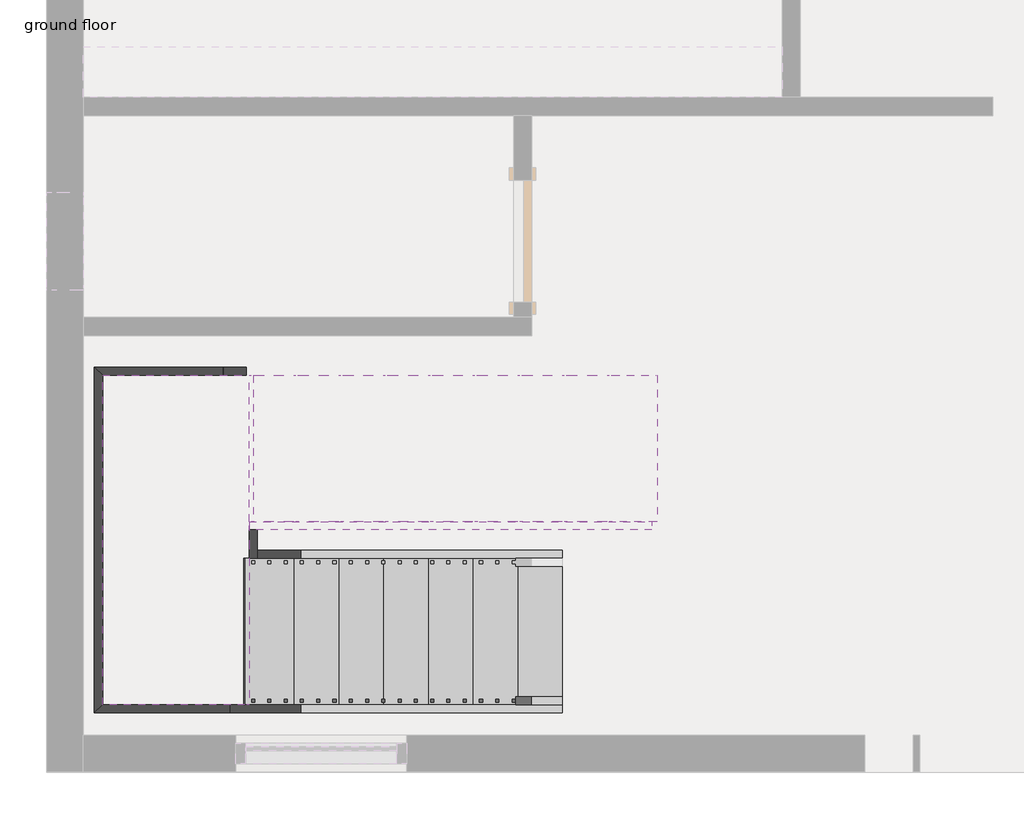
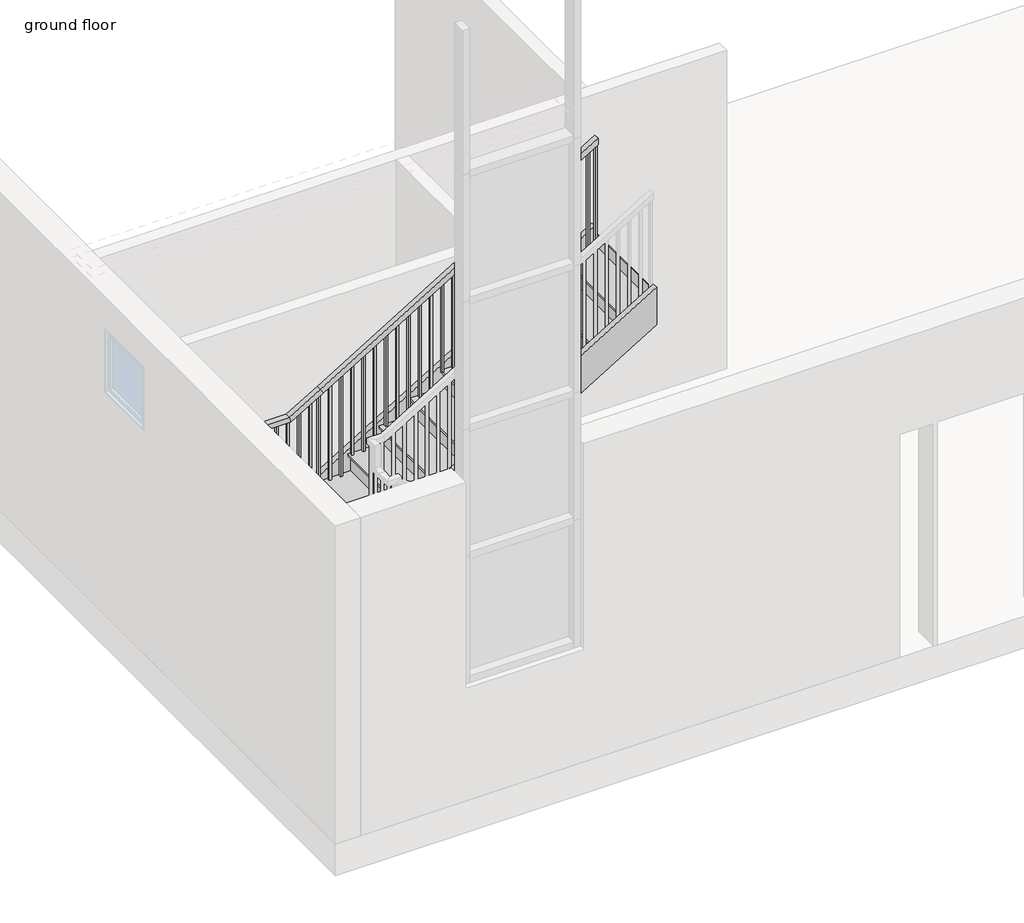
# One storey, part 3 of 3: 8 members, 2 stair flights, 1 railing, 1 slab.
"""IFC4 building model written with IfcOpenShell, lengths in millimetres."""

from ifc_helpers import new_model, si_unit, frame, origin, place, context, project, spatial, polyline, outline, extrude, faceted_brep, transform, mapped, element, save
from components import non_monolithic_landing_1e1f2eae, stair_flight_155d8820, stair_flight_d3a95e7b

model = new_model("IFC4")

# Units and contexts
model_context = context("Model", 3, world=origin())
ifc_project = project(units=[si_unit("LENGTHUNIT", "METRE", prefix="MILLI")], contexts=[model_context])

# Site, building, storey
site = spatial("IfcSite", under=ifc_project)
building = spatial("IfcBuilding", under=site)
storey = spatial("IfcBuildingStorey", under=building, Name="ground floor", Elevation=304.8)

# Members
placement = place(None, origin())
element("IfcMember", 1, ObjectType="Stringer - 2\" Width", at=placement, inside=storey, context=model_context, shape_type="SweptSolid", body=[
    extrude(outline(polyline([(304.8, -12620.1777023), (516.914512, -12620.1777023), (1735.6666667, -14631.1187576), (1430.8666667, -14716.2732141), (304.8, -12858.2632141), (304.8, -12620.1777023)])), frame((0.0, -405.7320925, 0.0), z_axis=(0.0, 1.0, 0.0), x_axis=(0.0, 0.0, 1.0)), (0.0, 0.0, 1.0), 50.8),
])
element("IfcMember", 2, ObjectType="Stringer - 2\" Width", at=placement, inside=storey, context=model_context, shape_type="SweptSolid", body=[
    extrude(outline(polyline([(304.8, -12620.1777023), (516.914512, -12620.1777023), (1671.4599665, -14525.1777023), (1315.051205, -14525.1777023), (304.8, -12858.2632141), (304.8, -12620.1777023)])), frame((0.0, 559.4679075, 0.0), z_axis=(0.0, 1.0, 0.0), x_axis=(0.0, 0.0, 1.0)), (0.0, 0.0, 1.0), 50.8),
])
element("IfcMember", 3, ObjectType="Stringer - 2\" Width", at=placement, inside=storey, context=model_context, shape_type="SweptSolid", body=[
    extrude(outline(polyline([(1735.6666667, -14800.2366471), (1430.8666667, -14715.0821905), (3039.1724171, -12061.3777023), (3395.5811786, -12061.3777023), (1735.6666667, -14800.2366471)])), frame((0.0, 1702.4679075, 0.0), z_axis=(0.0, 1.0, 0.0), x_axis=(0.0, 0.0, 1.0)), (0.0, 0.0, 1.0), 50.8),
])
element("IfcMember", 4, ObjectType="Stringer - 2\" Width", at=placement, inside=storey, context=model_context, shape_type="SweptSolid", body=[
    extrude(outline(polyline([(1871.5811786, -14575.9777023), (1515.1724171, -14575.9777023), (3039.1724171, -12061.3777023), (3395.5811786, -12061.3777023), (1871.5811786, -14575.9777023)])), frame((0.0, 737.2679075, 0.0), z_axis=(0.0, 1.0, 0.0), x_axis=(0.0, 0.0, 1.0)), (0.0, 0.0, 1.0), 50.8),
])
element("IfcMember", 5, ObjectType="Stringer - 2\" Width", at=placement, inside=storey, context=model_context, shape_type="Brep", body=[
    faceted_brep([(-14800.2366471, 1702.4679075, 1735.6666667), (-14800.2366471, 1753.2679075, 1735.6666667), (-15541.1777023, 1753.2679075, 1735.6666667), (-15490.3777023, 1702.4679075, 1735.6666667), (-14715.0821905, 1702.4679075, 1430.8666667), (-15490.3777023, 1702.4679075, 1430.8666667), (-14715.0821905, 1753.2679075, 1430.8666667), (-15541.1777023, 1753.2679075, 1430.8666667)], [[[0, 1, 2, 3]], [[4, 0, 3, 5]], [[6, 4, 5, 7]], [[1, 6, 7, 2]], [[1, 0, 4, 6]], [[2, 7, 5, 3]]]),
])
element("IfcMember", 6, ObjectType="Stringer - 2\" Width", at=placement, inside=storey, context=model_context, shape_type="SweptSolid", body=[
    extrude(outline(polyline([(-15541.1777023, 1753.2679075), (-15490.3777023, 1702.4679075), (-15490.3777023, -354.9320925), (-15541.1777023, -405.7320925), (-15541.1777023, 1753.2679075)])), frame((0.0, 0.0, 1430.8666667), z_axis=(0.0, 0.0, 1.0), x_axis=(1.0, 0.0, 0.0)), (0.0, 0.0, 1.0), 304.8),
])
element("IfcMember", 7, ObjectType="Stringer - 2\" Width", at=placement, inside=storey, context=model_context, shape_type="Brep", body=[
    faceted_brep([(-15490.3777023, -354.9320925, 1735.6666667), (-15541.1777023, -405.7320925, 1735.6666667), (-14631.1187576, -405.7320925, 1735.6666667), (-14631.1187576, -354.9320925, 1735.6666667), (-15490.3777023, -354.9320925, 1430.8666667), (-14716.2732141, -354.9320925, 1430.8666667), (-15541.1777023, -405.7320925, 1430.8666667), (-14716.2732141, -405.7320925, 1430.8666667)], [[[0, 1, 2, 3]], [[4, 0, 3, 5]], [[6, 4, 5, 7]], [[1, 6, 7, 2]], [[1, 0, 4, 6]], [[2, 7, 5, 3]]]),
])
element("IfcMember", 8, ObjectType="Stringer - 2\" Width", at=placement, inside=storey, context=model_context, shape_type="SweptSolid", body=[
    extrude(outline(polyline([(-14525.1777023, 559.4679075), (-14575.9777023, 559.4679075), (-14575.9777023, 737.2679075), (-14525.1777023, 737.2679075), (-14525.1777023, 559.4679075)])), frame((0.0, 0.0, 1430.8666667), z_axis=(0.0, 0.0, 1.0), x_axis=(1.0, 0.0, 0.0)), (0.0, 0.0, 1.0), 304.8),
])

# Railing
element("IfcRailing", 9, ObjectType="Handrail - Rectangular", at=placement, inside=storey, context=model_context, shape_type="SolidModel", body=[
    faceted_brep([(-12620.1777023, -354.9320925, 1388.5333333), (-12620.1777023, -354.9320925, 1329.1318731), (-12620.1777023, -304.1320925, 1329.1318731), (-12620.1777023, -304.1320925, 1388.5333333), (-14575.9777023, -354.9320925, 2573.8666667), (-14590.1701117, -354.9320925, 2523.0666667), (-14590.1701117, -304.1320925, 2523.0666667), (-14575.9777023, -304.1320925, 2573.8666667), (-15490.3777023, -354.9320925, 2573.8666667), (-15490.3777023, -354.9320925, 2523.0666667), (-15439.5777023, -304.1320925, 2523.0666667), (-15439.5777023, -304.1320925, 2573.8666667), (-15490.3777023, 1702.4679075, 2573.8666667), (-15490.3777023, 1702.4679075, 2523.0666667), (-15439.5777023, 1651.6679075, 2523.0666667), (-15439.5777023, 1651.6679075, 2573.8666667), (-14855.3777023, 1702.4679075, 2573.8666667), (-14841.1852929, 1702.4679075, 2523.0666667), (-14841.1852929, 1651.6679075, 2523.0666667), (-14855.3777023, 1651.6679075, 2573.8666667), (-14575.9777023, 1702.4679075, 2743.2), (-14549.6479751, 1702.4679075, 2699.7559502), (-14549.6479751, 1651.6679075, 2699.7559502), (-14575.9777023, 1651.6679075, 2743.2), (-12061.3777023, 1702.4679075, 4267.2), (-12061.3777023, 1651.6679075, 4267.2), (-12061.3777023, 1651.6679075, 4207.7985397), (-12061.3777023, 1702.4679075, 4207.7985397)], [[[0, 1, 2, 3]], [[1, 0, 4, 5]], [[2, 1, 5, 6]], [[3, 2, 6, 7]], [[0, 3, 7, 4]], [[5, 4, 8, 9]], [[6, 5, 9, 10]], [[7, 6, 10, 11]], [[4, 7, 11, 8]], [[9, 8, 12, 13]], [[10, 9, 13, 14]], [[11, 10, 14, 15]], [[8, 11, 15, 12]], [[13, 12, 16, 17]], [[14, 13, 17, 18]], [[15, 14, 18, 19]], [[12, 15, 19, 16]], [[17, 16, 20, 21]], [[18, 17, 21, 22]], [[19, 18, 22, 23]], [[16, 19, 23, 20]], [[24, 25, 26, 27]], [[21, 20, 24, 27]], [[22, 21, 27, 26]], [[23, 22, 26, 25]], [[20, 23, 25, 24]]]),
    extrude(outline(polyline([(4155.8439943, -12147.1027023), (3183.4666667, -12147.1027023), (3183.4666667, -12128.0527023), (4167.3894488, -12128.0527023), (4155.8439943, -12147.1027023)])), frame((0.0, 1667.5429075, 0.0), z_axis=(0.0, 1.0, 0.0), x_axis=(0.0, 0.0, 1.0)), (0.0, 0.0, 1.0), 19.05),
    extrude(outline(polyline([(4094.2682367, -12248.7027023), (3183.4666667, -12248.7027023), (3183.4666667, -12229.6527023), (4105.8136913, -12229.6527023), (4094.2682367, -12248.7027023)])), frame((0.0, 1667.5429075, 0.0), z_axis=(0.0, 1.0, 0.0), x_axis=(0.0, 0.0, 1.0)), (0.0, 0.0, 1.0), 19.05),
    extrude(outline(polyline([(4032.6924791, -12350.3027023), (3183.4666667, -12350.3027023), (3183.4666667, -12331.2527023), (4044.2379337, -12331.2527023), (4032.6924791, -12350.3027023)])), frame((0.0, 1667.5429075, 0.0), z_axis=(0.0, 1.0, 0.0), x_axis=(0.0, 0.0, 1.0)), (0.0, 0.0, 1.0), 19.05),
    extrude(outline(polyline([(3971.1167216, -12451.9027023), (3014.1333333, -12451.9027023), (3014.1333333, -12432.8527023), (3982.6621761, -12432.8527023), (3971.1167216, -12451.9027023)])), frame((0.0, 1667.5429075, 0.0), z_axis=(0.0, 1.0, 0.0), x_axis=(0.0, 0.0, 1.0)), (0.0, 0.0, 1.0), 19.05),
    extrude(outline(polyline([(3909.540964, -12553.5027023), (3014.1333333, -12553.5027023), (3014.1333333, -12534.4527023), (3921.0864185, -12534.4527023), (3909.540964, -12553.5027023)])), frame((0.0, 1667.5429075, 0.0), z_axis=(0.0, 1.0, 0.0), x_axis=(0.0, 0.0, 1.0)), (0.0, 0.0, 1.0), 19.05),
    extrude(outline(polyline([(3847.9652064, -12655.1027023), (2844.8, -12655.1027023), (2844.8, -12636.0527023), (3859.510661, -12636.0527023), (3847.9652064, -12655.1027023)])), frame((0.0, 1667.5429075, 0.0), z_axis=(0.0, 1.0, 0.0), x_axis=(0.0, 0.0, 1.0)), (0.0, 0.0, 1.0), 19.05),
    extrude(outline(polyline([(3786.3894488, -12756.7027023), (2844.8, -12756.7027023), (2844.8, -12737.6527023), (3797.9349034, -12737.6527023), (3786.3894488, -12756.7027023)])), frame((0.0, 1667.5429075, 0.0), z_axis=(0.0, 1.0, 0.0), x_axis=(0.0, 0.0, 1.0)), (0.0, 0.0, 1.0), 19.05),
    extrude(outline(polyline([(3724.8136913, -12858.3027023), (2844.8, -12858.3027023), (2844.8, -12839.2527023), (3736.3591458, -12839.2527023), (3724.8136913, -12858.3027023)])), frame((0.0, 1667.5429075, 0.0), z_axis=(0.0, 1.0, 0.0), x_axis=(0.0, 0.0, 1.0)), (0.0, 0.0, 1.0), 19.05),
    extrude(outline(polyline([(3663.2379337, -12959.9027023), (2675.4666667, -12959.9027023), (2675.4666667, -12940.8527023), (3674.7833882, -12940.8527023), (3663.2379337, -12959.9027023)])), frame((0.0, 1667.5429075, 0.0), z_axis=(0.0, 1.0, 0.0), x_axis=(0.0, 0.0, 1.0)), (0.0, 0.0, 1.0), 19.05),
    extrude(outline(polyline([(3601.6621761, -13061.5027023), (2675.4666667, -13061.5027023), (2675.4666667, -13042.4527023), (3613.2076307, -13042.4527023), (3601.6621761, -13061.5027023)])), frame((0.0, 1667.5429075, 0.0), z_axis=(0.0, 1.0, 0.0), x_axis=(0.0, 0.0, 1.0)), (0.0, 0.0, 1.0), 19.05),
    extrude(outline(polyline([(3540.0864185, -13163.1027023), (2675.4666667, -13163.1027023), (2675.4666667, -13144.0527023), (3551.6318731, -13144.0527023), (3540.0864185, -13163.1027023)])), frame((0.0, 1667.5429075, 0.0), z_axis=(0.0, 1.0, 0.0), x_axis=(0.0, 0.0, 1.0)), (0.0, 0.0, 1.0), 19.05),
    extrude(outline(polyline([(3478.510661, -13264.7027023), (2506.1333333, -13264.7027023), (2506.1333333, -13245.6527023), (3490.0561155, -13245.6527023), (3478.510661, -13264.7027023)])), frame((0.0, 1667.5429075, 0.0), z_axis=(0.0, 1.0, 0.0), x_axis=(0.0, 0.0, 1.0)), (0.0, 0.0, 1.0), 19.05),
    extrude(outline(polyline([(3416.9349034, -13366.3027023), (2506.1333333, -13366.3027023), (2506.1333333, -13347.2527023), (3428.4803579, -13347.2527023), (3416.9349034, -13366.3027023)])), frame((0.0, 1667.5429075, 0.0), z_axis=(0.0, 1.0, 0.0), x_axis=(0.0, 0.0, 1.0)), (0.0, 0.0, 1.0), 19.05),
    extrude(outline(polyline([(3355.3591458, -13467.9027023), (2506.1333333, -13467.9027023), (2506.1333333, -13448.8527023), (3366.9046004, -13448.8527023), (3355.3591458, -13467.9027023)])), frame((0.0, 1667.5429075, 0.0), z_axis=(0.0, 1.0, 0.0), x_axis=(0.0, 0.0, 1.0)), (0.0, 0.0, 1.0), 19.05),
    extrude(outline(polyline([(3293.7833882, -13569.5027023), (2336.8, -13569.5027023), (2336.8, -13550.4527023), (3305.3288428, -13550.4527023), (3293.7833882, -13569.5027023)])), frame((0.0, 1667.5429075, 0.0), z_axis=(0.0, 1.0, 0.0), x_axis=(0.0, 0.0, 1.0)), (0.0, 0.0, 1.0), 19.05),
    extrude(outline(polyline([(3232.2076307, -13671.1027023), (2336.8, -13671.1027023), (2336.8, -13652.0527023), (3243.7530852, -13652.0527023), (3232.2076307, -13671.1027023)])), frame((0.0, 1667.5429075, 0.0), z_axis=(0.0, 1.0, 0.0), x_axis=(0.0, 0.0, 1.0)), (0.0, 0.0, 1.0), 19.05),
    extrude(outline(polyline([(3170.6318731, -13772.7027023), (2167.4666667, -13772.7027023), (2167.4666667, -13753.6527023), (3182.1773276, -13753.6527023), (3170.6318731, -13772.7027023)])), frame((0.0, 1667.5429075, 0.0), z_axis=(0.0, 1.0, 0.0), x_axis=(0.0, 0.0, 1.0)), (0.0, 0.0, 1.0), 19.05),
    extrude(outline(polyline([(3109.0561155, -13874.3027023), (2167.4666667, -13874.3027023), (2167.4666667, -13855.2527023), (3120.60157, -13855.2527023), (3109.0561155, -13874.3027023)])), frame((0.0, 1667.5429075, 0.0), z_axis=(0.0, 1.0, 0.0), x_axis=(0.0, 0.0, 1.0)), (0.0, 0.0, 1.0), 19.05),
    extrude(outline(polyline([(3047.4803579, -13975.9027023), (2167.4666667, -13975.9027023), (2167.4666667, -13956.8527023), (3059.0258125, -13956.8527023), (3047.4803579, -13975.9027023)])), frame((0.0, 1667.5429075, 0.0), z_axis=(0.0, 1.0, 0.0), x_axis=(0.0, 0.0, 1.0)), (0.0, 0.0, 1.0), 19.05),
    extrude(outline(polyline([(2985.9046004, -14077.5027023), (1998.1333333, -14077.5027023), (1998.1333333, -14058.4527023), (2997.4500549, -14058.4527023), (2985.9046004, -14077.5027023)])), frame((0.0, 1667.5429075, 0.0), z_axis=(0.0, 1.0, 0.0), x_axis=(0.0, 0.0, 1.0)), (0.0, 0.0, 1.0), 19.05),
    extrude(outline(polyline([(2924.3288428, -14179.1027023), (1998.1333333, -14179.1027023), (1998.1333333, -14160.0527023), (2935.8742973, -14160.0527023), (2924.3288428, -14179.1027023)])), frame((0.0, 1667.5429075, 0.0), z_axis=(0.0, 1.0, 0.0), x_axis=(0.0, 0.0, 1.0)), (0.0, 0.0, 1.0), 19.05),
    extrude(outline(polyline([(2862.7530852, -14280.7027023), (1998.1333333, -14280.7027023), (1998.1333333, -14261.6527023), (2874.2985397, -14261.6527023), (2862.7530852, -14280.7027023)])), frame((0.0, 1667.5429075, 0.0), z_axis=(0.0, 1.0, 0.0), x_axis=(0.0, 0.0, 1.0)), (0.0, 0.0, 1.0), 19.05),
    extrude(outline(polyline([(2801.1773276, -14382.3027023), (1828.8, -14382.3027023), (1828.8, -14363.2527023), (2812.7227822, -14363.2527023), (2801.1773276, -14382.3027023)])), frame((0.0, 1667.5429075, 0.0), z_axis=(0.0, 1.0, 0.0), x_axis=(0.0, 0.0, 1.0)), (0.0, 0.0, 1.0), 19.05),
    extrude(outline(polyline([(2739.60157, -14483.9027023), (1828.8, -14483.9027023), (1828.8, -14464.8527023), (2751.1470246, -14464.8527023), (2739.60157, -14483.9027023)])), frame((0.0, 1667.5429075, 0.0), z_axis=(0.0, 1.0, 0.0), x_axis=(0.0, 0.0, 1.0)), (0.0, 0.0, 1.0), 19.05),
    extrude(outline(polyline([(2631.8439943, -14661.7027023), (1659.4666667, -14661.7027023), (1659.4666667, -14642.6527023), (2643.3894488, -14642.6527023), (2631.8439943, -14661.7027023)])), frame((0.0, 1667.5429075, 0.0), z_axis=(0.0, 1.0, 0.0), x_axis=(0.0, 0.0, 1.0)), (0.0, 0.0, 1.0), 19.05),
    extrude(outline(polyline([(2570.2682367, -14763.3027023), (1659.4666667, -14763.3027023), (1659.4666667, -14744.2527023), (2581.8136913, -14744.2527023), (2570.2682367, -14763.3027023)])), frame((0.0, 1667.5429075, 0.0), z_axis=(0.0, 1.0, 0.0), x_axis=(0.0, 0.0, 1.0)), (0.0, 0.0, 1.0), 19.05),
    extrude(outline(polyline([(-14864.9027023, 1686.5929075), (-14845.8527023, 1686.5929075), (-14845.8527023, 1667.5429075), (-14864.9027023, 1667.5429075), (-14864.9027023, 1686.5929075)])), frame((0.0, 0.0, 1659.4666667), z_axis=(0.0, 0.0, 1.0), x_axis=(1.0, 0.0, 0.0)), (0.0, 0.0, 1.0), 863.6),
    extrude(outline(polyline([(-14966.5027023, 1686.5929075), (-14947.4527023, 1686.5929075), (-14947.4527023, 1667.5429075), (-14966.5027023, 1667.5429075), (-14966.5027023, 1686.5929075)])), frame((0.0, 0.0, 1659.4666667), z_axis=(0.0, 0.0, 1.0), x_axis=(1.0, 0.0, 0.0)), (0.0, 0.0, 1.0), 863.6),
    extrude(outline(polyline([(-15068.1027023, 1686.5929075), (-15049.0527023, 1686.5929075), (-15049.0527023, 1667.5429075), (-15068.1027023, 1667.5429075), (-15068.1027023, 1686.5929075)])), frame((0.0, 0.0, 1659.4666667), z_axis=(0.0, 0.0, 1.0), x_axis=(1.0, 0.0, 0.0)), (0.0, 0.0, 1.0), 863.6),
    extrude(outline(polyline([(-15169.7027023, 1686.5929075), (-15150.6527023, 1686.5929075), (-15150.6527023, 1667.5429075), (-15169.7027023, 1667.5429075), (-15169.7027023, 1686.5929075)])), frame((0.0, 0.0, 1659.4666667), z_axis=(0.0, 0.0, 1.0), x_axis=(1.0, 0.0, 0.0)), (0.0, 0.0, 1.0), 863.6),
    extrude(outline(polyline([(-15271.3027023, 1686.5929075), (-15252.2527023, 1686.5929075), (-15252.2527023, 1667.5429075), (-15271.3027023, 1667.5429075), (-15271.3027023, 1686.5929075)])), frame((0.0, 0.0, 1659.4666667), z_axis=(0.0, 0.0, 1.0), x_axis=(1.0, 0.0, 0.0)), (0.0, 0.0, 1.0), 863.6),
    extrude(outline(polyline([(-15372.9027023, 1686.5929075), (-15353.8527023, 1686.5929075), (-15353.8527023, 1667.5429075), (-15372.9027023, 1667.5429075), (-15372.9027023, 1686.5929075)])), frame((0.0, 0.0, 1659.4666667), z_axis=(0.0, 0.0, 1.0), x_axis=(1.0, 0.0, 0.0)), (0.0, 0.0, 1.0), 863.6),
    extrude(outline(polyline([(-15474.5027023, 1591.3429075), (-15474.5027023, 1610.3929075), (-15455.4527023, 1610.3929075), (-15455.4527023, 1591.3429075), (-15474.5027023, 1591.3429075)])), frame((0.0, 0.0, 1659.4666667), z_axis=(0.0, 0.0, 1.0), x_axis=(1.0, 0.0, 0.0)), (0.0, 0.0, 1.0), 863.6),
    extrude(outline(polyline([(-15474.5027023, 1489.7429075), (-15474.5027023, 1508.7929075), (-15455.4527023, 1508.7929075), (-15455.4527023, 1489.7429075), (-15474.5027023, 1489.7429075)])), frame((0.0, 0.0, 1659.4666667), z_axis=(0.0, 0.0, 1.0), x_axis=(1.0, 0.0, 0.0)), (0.0, 0.0, 1.0), 863.6),
    extrude(outline(polyline([(-15474.5027023, 1388.1429075), (-15474.5027023, 1407.1929075), (-15455.4527023, 1407.1929075), (-15455.4527023, 1388.1429075), (-15474.5027023, 1388.1429075)])), frame((0.0, 0.0, 1659.4666667), z_axis=(0.0, 0.0, 1.0), x_axis=(1.0, 0.0, 0.0)), (0.0, 0.0, 1.0), 863.6),
    extrude(outline(polyline([(-15474.5027023, 1286.5429075), (-15474.5027023, 1305.5929075), (-15455.4527023, 1305.5929075), (-15455.4527023, 1286.5429075), (-15474.5027023, 1286.5429075)])), frame((0.0, 0.0, 1659.4666667), z_axis=(0.0, 0.0, 1.0), x_axis=(1.0, 0.0, 0.0)), (0.0, 0.0, 1.0), 863.6),
    extrude(outline(polyline([(-15474.5027023, 1184.9429075), (-15474.5027023, 1203.9929075), (-15455.4527023, 1203.9929075), (-15455.4527023, 1184.9429075), (-15474.5027023, 1184.9429075)])), frame((0.0, 0.0, 1659.4666667), z_axis=(0.0, 0.0, 1.0), x_axis=(1.0, 0.0, 0.0)), (0.0, 0.0, 1.0), 863.6),
    extrude(outline(polyline([(-15474.5027023, 1083.3429075), (-15474.5027023, 1102.3929075), (-15455.4527023, 1102.3929075), (-15455.4527023, 1083.3429075), (-15474.5027023, 1083.3429075)])), frame((0.0, 0.0, 1659.4666667), z_axis=(0.0, 0.0, 1.0), x_axis=(1.0, 0.0, 0.0)), (0.0, 0.0, 1.0), 863.6),
    extrude(outline(polyline([(-15474.5027023, 981.7429075), (-15474.5027023, 1000.7929075), (-15455.4527023, 1000.7929075), (-15455.4527023, 981.7429075), (-15474.5027023, 981.7429075)])), frame((0.0, 0.0, 1659.4666667), z_axis=(0.0, 0.0, 1.0), x_axis=(1.0, 0.0, 0.0)), (0.0, 0.0, 1.0), 863.6),
    extrude(outline(polyline([(-15474.5027023, 880.1429075), (-15474.5027023, 899.1929075), (-15455.4527023, 899.1929075), (-15455.4527023, 880.1429075), (-15474.5027023, 880.1429075)])), frame((0.0, 0.0, 1659.4666667), z_axis=(0.0, 0.0, 1.0), x_axis=(1.0, 0.0, 0.0)), (0.0, 0.0, 1.0), 863.6),
    extrude(outline(polyline([(-15474.5027023, 778.5429075), (-15474.5027023, 797.5929075), (-15455.4527023, 797.5929075), (-15455.4527023, 778.5429075), (-15474.5027023, 778.5429075)])), frame((0.0, 0.0, 1659.4666667), z_axis=(0.0, 0.0, 1.0), x_axis=(1.0, 0.0, 0.0)), (0.0, 0.0, 1.0), 863.6),
    extrude(outline(polyline([(-15474.5027023, 676.9429075), (-15474.5027023, 695.9929075), (-15455.4527023, 695.9929075), (-15455.4527023, 676.9429075), (-15474.5027023, 676.9429075)])), frame((0.0, 0.0, 1659.4666667), z_axis=(0.0, 0.0, 1.0), x_axis=(1.0, 0.0, 0.0)), (0.0, 0.0, 1.0), 863.6),
    extrude(outline(polyline([(-15474.5027023, 575.3429075), (-15474.5027023, 594.3929075), (-15455.4527023, 594.3929075), (-15455.4527023, 575.3429075), (-15474.5027023, 575.3429075)])), frame((0.0, 0.0, 1659.4666667), z_axis=(0.0, 0.0, 1.0), x_axis=(1.0, 0.0, 0.0)), (0.0, 0.0, 1.0), 863.6),
    extrude(outline(polyline([(-15474.5027023, 473.7429075), (-15474.5027023, 492.7929075), (-15455.4527023, 492.7929075), (-15455.4527023, 473.7429075), (-15474.5027023, 473.7429075)])), frame((0.0, 0.0, 1659.4666667), z_axis=(0.0, 0.0, 1.0), x_axis=(1.0, 0.0, 0.0)), (0.0, 0.0, 1.0), 863.6),
    extrude(outline(polyline([(-15474.5027023, 372.1429075), (-15474.5027023, 391.1929075), (-15455.4527023, 391.1929075), (-15455.4527023, 372.1429075), (-15474.5027023, 372.1429075)])), frame((0.0, 0.0, 1659.4666667), z_axis=(0.0, 0.0, 1.0), x_axis=(1.0, 0.0, 0.0)), (0.0, 0.0, 1.0), 863.6),
    extrude(outline(polyline([(-15474.5027023, 270.5429075), (-15474.5027023, 289.5929075), (-15455.4527023, 289.5929075), (-15455.4527023, 270.5429075), (-15474.5027023, 270.5429075)])), frame((0.0, 0.0, 1659.4666667), z_axis=(0.0, 0.0, 1.0), x_axis=(1.0, 0.0, 0.0)), (0.0, 0.0, 1.0), 863.6),
    extrude(outline(polyline([(-15474.5027023, 168.9429075), (-15474.5027023, 187.9929075), (-15455.4527023, 187.9929075), (-15455.4527023, 168.9429075), (-15474.5027023, 168.9429075)])), frame((0.0, 0.0, 1659.4666667), z_axis=(0.0, 0.0, 1.0), x_axis=(1.0, 0.0, 0.0)), (0.0, 0.0, 1.0), 863.6),
    extrude(outline(polyline([(-15474.5027023, 67.3429075), (-15474.5027023, 86.3929075), (-15455.4527023, 86.3929075), (-15455.4527023, 67.3429075), (-15474.5027023, 67.3429075)])), frame((0.0, 0.0, 1659.4666667), z_axis=(0.0, 0.0, 1.0), x_axis=(1.0, 0.0, 0.0)), (0.0, 0.0, 1.0), 863.6),
    extrude(outline(polyline([(-15474.5027023, -34.2570925), (-15474.5027023, -15.2070925), (-15455.4527023, -15.2070925), (-15455.4527023, -34.2570925), (-15474.5027023, -34.2570925)])), frame((0.0, 0.0, 1659.4666667), z_axis=(0.0, 0.0, 1.0), x_axis=(1.0, 0.0, 0.0)), (0.0, 0.0, 1.0), 863.6),
    extrude(outline(polyline([(-15474.5027023, -135.8570925), (-15474.5027023, -116.8070925), (-15455.4527023, -116.8070925), (-15455.4527023, -135.8570925), (-15474.5027023, -135.8570925)])), frame((0.0, 0.0, 1659.4666667), z_axis=(0.0, 0.0, 1.0), x_axis=(1.0, 0.0, 0.0)), (0.0, 0.0, 1.0), 863.6),
    extrude(outline(polyline([(-15474.5027023, -237.4570925), (-15474.5027023, -218.4070925), (-15455.4527023, -218.4070925), (-15455.4527023, -237.4570925), (-15474.5027023, -237.4570925)])), frame((0.0, 0.0, 1659.4666667), z_axis=(0.0, 0.0, 1.0), x_axis=(1.0, 0.0, 0.0)), (0.0, 0.0, 1.0), 863.6),
    extrude(outline(polyline([(-15379.2527023, -339.0570925), (-15398.3027023, -339.0570925), (-15398.3027023, -320.0070925), (-15379.2527023, -320.0070925), (-15379.2527023, -339.0570925)])), frame((0.0, 0.0, 1659.4666667), z_axis=(0.0, 0.0, 1.0), x_axis=(1.0, 0.0, 0.0)), (0.0, 0.0, 1.0), 863.6),
    extrude(outline(polyline([(-15277.6527023, -339.0570925), (-15296.7027023, -339.0570925), (-15296.7027023, -320.0070925), (-15277.6527023, -320.0070925), (-15277.6527023, -339.0570925)])), frame((0.0, 0.0, 1659.4666667), z_axis=(0.0, 0.0, 1.0), x_axis=(1.0, 0.0, 0.0)), (0.0, 0.0, 1.0), 863.6),
    extrude(outline(polyline([(-15176.0527023, -339.0570925), (-15195.1027023, -339.0570925), (-15195.1027023, -320.0070925), (-15176.0527023, -320.0070925), (-15176.0527023, -339.0570925)])), frame((0.0, 0.0, 1659.4666667), z_axis=(0.0, 0.0, 1.0), x_axis=(1.0, 0.0, 0.0)), (0.0, 0.0, 1.0), 863.6),
    extrude(outline(polyline([(-15074.4527023, -339.0570925), (-15093.5027023, -339.0570925), (-15093.5027023, -320.0070925), (-15074.4527023, -320.0070925), (-15074.4527023, -339.0570925)])), frame((0.0, 0.0, 1659.4666667), z_axis=(0.0, 0.0, 1.0), x_axis=(1.0, 0.0, 0.0)), (0.0, 0.0, 1.0), 863.6),
    extrude(outline(polyline([(-14972.8527023, -339.0570925), (-14991.9027023, -339.0570925), (-14991.9027023, -320.0070925), (-14972.8527023, -320.0070925), (-14972.8527023, -339.0570925)])), frame((0.0, 0.0, 1659.4666667), z_axis=(0.0, 0.0, 1.0), x_axis=(1.0, 0.0, 0.0)), (0.0, 0.0, 1.0), 863.6),
    extrude(outline(polyline([(-14871.2527023, -339.0570925), (-14890.3027023, -339.0570925), (-14890.3027023, -320.0070925), (-14871.2527023, -320.0070925), (-14871.2527023, -339.0570925)])), frame((0.0, 0.0, 1659.4666667), z_axis=(0.0, 0.0, 1.0), x_axis=(1.0, 0.0, 0.0)), (0.0, 0.0, 1.0), 863.6),
    extrude(outline(polyline([(-14769.6527023, -339.0570925), (-14788.7027023, -339.0570925), (-14788.7027023, -320.0070925), (-14769.6527023, -320.0070925), (-14769.6527023, -339.0570925)])), frame((0.0, 0.0, 1659.4666667), z_axis=(0.0, 0.0, 1.0), x_axis=(1.0, 0.0, 0.0)), (0.0, 0.0, 1.0), 863.6),
    extrude(outline(polyline([(-14668.0527023, -339.0570925), (-14687.1027023, -339.0570925), (-14687.1027023, -320.0070925), (-14668.0527023, -320.0070925), (-14668.0527023, -339.0570925)])), frame((0.0, 0.0, 1659.4666667), z_axis=(0.0, 0.0, 1.0), x_axis=(1.0, 0.0, 0.0)), (0.0, 0.0, 1.0), 863.6),
    extrude(outline(polyline([(2504.8439943, -14560.1027023), (1490.1333333, -14560.1027023), (1490.1333333, -14541.0527023), (2493.2985397, -14541.0527023), (2504.8439943, -14560.1027023)])), frame((0.0, -339.0570925, 0.0), z_axis=(0.0, 1.0, 0.0), x_axis=(0.0, 0.0, 1.0)), (0.0, 0.0, 1.0), 19.05),
    extrude(outline(polyline([(2443.2682367, -14458.5027023), (1490.1333333, -14458.5027023), (1490.1333333, -14439.4527023), (2431.7227822, -14439.4527023), (2443.2682367, -14458.5027023)])), frame((0.0, -339.0570925, 0.0), z_axis=(0.0, 1.0, 0.0), x_axis=(0.0, 0.0, 1.0)), (0.0, 0.0, 1.0), 19.05),
    extrude(outline(polyline([(2381.6924791, -14356.9027023), (1490.1333333, -14356.9027023), (1490.1333333, -14337.8527023), (2370.1470246, -14337.8527023), (2381.6924791, -14356.9027023)])), frame((0.0, -339.0570925, 0.0), z_axis=(0.0, 1.0, 0.0), x_axis=(0.0, 0.0, 1.0)), (0.0, 0.0, 1.0), 19.05),
    extrude(outline(polyline([(2320.1167216, -14255.3027023), (1320.8, -14255.3027023), (1320.8, -14236.2527023), (2308.571267, -14236.2527023), (2320.1167216, -14255.3027023)])), frame((0.0, -339.0570925, 0.0), z_axis=(0.0, 1.0, 0.0), x_axis=(0.0, 0.0, 1.0)), (0.0, 0.0, 1.0), 19.05),
    extrude(outline(polyline([(2258.540964, -14153.7027023), (1320.8, -14153.7027023), (1320.8, -14134.6527023), (2246.9955094, -14134.6527023), (2258.540964, -14153.7027023)])), frame((0.0, -339.0570925, 0.0), z_axis=(0.0, 1.0, 0.0), x_axis=(0.0, 0.0, 1.0)), (0.0, 0.0, 1.0), 19.05),
    extrude(outline(polyline([(2196.9652064, -14052.1027023), (1320.8, -14052.1027023), (1320.8, -14033.0527023), (2185.4197519, -14033.0527023), (2196.9652064, -14052.1027023)])), frame((0.0, -339.0570925, 0.0), z_axis=(0.0, 1.0, 0.0), x_axis=(0.0, 0.0, 1.0)), (0.0, 0.0, 1.0), 19.05),
    extrude(outline(polyline([(2135.3894488, -13950.5027023), (1151.4666667, -13950.5027023), (1151.4666667, -13931.4527023), (2123.8439943, -13931.4527023), (2135.3894488, -13950.5027023)])), frame((0.0, -339.0570925, 0.0), z_axis=(0.0, 1.0, 0.0), x_axis=(0.0, 0.0, 1.0)), (0.0, 0.0, 1.0), 19.05),
    extrude(outline(polyline([(2073.8136913, -13848.9027023), (1151.4666667, -13848.9027023), (1151.4666667, -13829.8527023), (2062.2682367, -13829.8527023), (2073.8136913, -13848.9027023)])), frame((0.0, -339.0570925, 0.0), z_axis=(0.0, 1.0, 0.0), x_axis=(0.0, 0.0, 1.0)), (0.0, 0.0, 1.0), 19.05),
    extrude(outline(polyline([(2012.2379337, -13747.3027023), (1151.4666667, -13747.3027023), (1151.4666667, -13728.2527023), (2000.6924791, -13728.2527023), (2012.2379337, -13747.3027023)])), frame((0.0, -339.0570925, 0.0), z_axis=(0.0, 1.0, 0.0), x_axis=(0.0, 0.0, 1.0)), (0.0, 0.0, 1.0), 19.05),
    extrude(outline(polyline([(1950.6621761, -13645.7027023), (982.1333333, -13645.7027023), (982.1333333, -13626.6527023), (1939.1167216, -13626.6527023), (1950.6621761, -13645.7027023)])), frame((0.0, -339.0570925, 0.0), z_axis=(0.0, 1.0, 0.0), x_axis=(0.0, 0.0, 1.0)), (0.0, 0.0, 1.0), 19.05),
    extrude(outline(polyline([(1889.0864185, -13544.1027023), (982.1333333, -13544.1027023), (982.1333333, -13525.0527023), (1877.540964, -13525.0527023), (1889.0864185, -13544.1027023)])), frame((0.0, -339.0570925, 0.0), z_axis=(0.0, 1.0, 0.0), x_axis=(0.0, 0.0, 1.0)), (0.0, 0.0, 1.0), 19.05),
    extrude(outline(polyline([(1827.510661, -13442.5027023), (812.8, -13442.5027023), (812.8, -13423.4527023), (1815.9652064, -13423.4527023), (1827.510661, -13442.5027023)])), frame((0.0, -339.0570925, 0.0), z_axis=(0.0, 1.0, 0.0), x_axis=(0.0, 0.0, 1.0)), (0.0, 0.0, 1.0), 19.05),
    extrude(outline(polyline([(1765.9349034, -13340.9027023), (812.8, -13340.9027023), (812.8, -13321.8527023), (1754.3894488, -13321.8527023), (1765.9349034, -13340.9027023)])), frame((0.0, -339.0570925, 0.0), z_axis=(0.0, 1.0, 0.0), x_axis=(0.0, 0.0, 1.0)), (0.0, 0.0, 1.0), 19.05),
    extrude(outline(polyline([(1704.3591458, -13239.3027023), (812.8, -13239.3027023), (812.8, -13220.2527023), (1692.8136913, -13220.2527023), (1704.3591458, -13239.3027023)])), frame((0.0, -339.0570925, 0.0), z_axis=(0.0, 1.0, 0.0), x_axis=(0.0, 0.0, 1.0)), (0.0, 0.0, 1.0), 19.05),
    extrude(outline(polyline([(1642.7833882, -13137.7027023), (643.4666667, -13137.7027023), (643.4666667, -13118.6527023), (1631.2379337, -13118.6527023), (1642.7833882, -13137.7027023)])), frame((0.0, -339.0570925, 0.0), z_axis=(0.0, 1.0, 0.0), x_axis=(0.0, 0.0, 1.0)), (0.0, 0.0, 1.0), 19.05),
    extrude(outline(polyline([(1581.2076307, -13036.1027023), (643.4666667, -13036.1027023), (643.4666667, -13017.0527023), (1569.6621761, -13017.0527023), (1581.2076307, -13036.1027023)])), frame((0.0, -339.0570925, 0.0), z_axis=(0.0, 1.0, 0.0), x_axis=(0.0, 0.0, 1.0)), (0.0, 0.0, 1.0), 19.05),
    extrude(outline(polyline([(1519.6318731, -12934.5027023), (643.4666667, -12934.5027023), (643.4666667, -12915.4527023), (1508.0864185, -12915.4527023), (1519.6318731, -12934.5027023)])), frame((0.0, -339.0570925, 0.0), z_axis=(0.0, 1.0, 0.0), x_axis=(0.0, 0.0, 1.0)), (0.0, 0.0, 1.0), 19.05),
    extrude(outline(polyline([(1458.0561155, -12832.9027023), (474.1333333, -12832.9027023), (474.1333333, -12813.8527023), (1446.510661, -12813.8527023), (1458.0561155, -12832.9027023)])), frame((0.0, -339.0570925, 0.0), z_axis=(0.0, 1.0, 0.0), x_axis=(0.0, 0.0, 1.0)), (0.0, 0.0, 1.0), 19.05),
    extrude(outline(polyline([(1396.4803579, -12731.3027023), (474.1333333, -12731.3027023), (474.1333333, -12712.2527023), (1384.9349034, -12712.2527023), (1396.4803579, -12731.3027023)])), frame((0.0, -339.0570925, 0.0), z_axis=(0.0, 1.0, 0.0), x_axis=(0.0, 0.0, 1.0)), (0.0, 0.0, 1.0), 19.05),
    extrude(outline(polyline([(2678.0258125, -14585.5027023), (1659.4666667, -14585.5027023), (1659.4666667, -14566.4527023), (2689.571267, -14566.4527023), (2678.0258125, -14585.5027023)])), frame((0.0, 1667.5429075, 0.0), z_axis=(0.0, 1.0, 0.0), x_axis=(0.0, 0.0, 1.0)), (0.0, 0.0, 1.0), 19.05),
    extrude(outline(polyline([(-15474.5027023, 1667.5429075), (-15474.5027023, 1686.5929075), (-15455.4527023, 1686.5929075), (-15455.4527023, 1667.5429075), (-15474.5027023, 1667.5429075)])), frame((0.0, 0.0, 1659.4666667), z_axis=(0.0, 0.0, 1.0), x_axis=(1.0, 0.0, 0.0)), (0.0, 0.0, 1.0), 863.6),
    extrude(outline(polyline([(-15455.4527023, -339.0570925), (-15474.5027023, -339.0570925), (-15474.5027023, -320.0070925), (-15455.4527023, -320.0070925), (-15455.4527023, -339.0570925)])), frame((0.0, 0.0, 1659.4666667), z_axis=(0.0, 0.0, 1.0), x_axis=(1.0, 0.0, 0.0)), (0.0, 0.0, 1.0), 863.6),
    extrude(outline(polyline([(2520.2379337, -14585.5027023), (1659.4666667, -14585.5027023), (1659.4666667, -14566.4527023), (2508.6924791, -14566.4527023), (2520.2379337, -14585.5027023)])), frame((0.0, -339.0570925, 0.0), z_axis=(0.0, 1.0, 0.0), x_axis=(0.0, 0.0, 1.0)), (0.0, 0.0, 1.0), 19.05),
    extrude(outline(polyline([(4196.2530852, -12080.4277023), (3183.4666667, -12080.4277023), (3183.4666667, -12061.3777023), (4207.7985397, -12061.3777023), (4196.2530852, -12080.4277023)])), frame((0.0, 1667.5429075, 0.0), z_axis=(0.0, 1.0, 0.0), x_axis=(0.0, 0.0, 1.0)), (0.0, 0.0, 1.0), 19.05),
    extrude(outline(polyline([(1340.6773276, -12639.2277023), (474.1333333, -12639.2277023), (474.1333333, -12620.1777023), (1329.1318731, -12620.1777023), (1340.6773276, -12639.2277023)])), frame((0.0, -339.0570925, 0.0), z_axis=(0.0, 1.0, 0.0), x_axis=(0.0, 0.0, 1.0)), (0.0, 0.0, 1.0), 19.05),
])

# Slab
non_monolithic_landing_shape = non_monolithic_landing_1e1f2eae(model_context)
element("IfcSlab", 10, ObjectType="Non-Monolithic Landing", at=placement, inside=storey, context=model_context, shape_type="MappedRepresentation", body=[
    mapped(non_monolithic_landing_shape, transform((0.0, 0.0, 0.0), x_axis=(1.0, 0.0, 0.0), y_axis=(0.0, 1.0, 0.0), z_axis=(0.0, 0.0, 1.0))),
])

# Stair flights
stair_flight_shape = stair_flight_155d8820(model_context)
element("IfcStairFlight", 11, ObjectType="2\" Tread 1\" Nosing 1/4\" Riser", at=placement, inside=storey, context=model_context, shape_type="MappedRepresentation", body=[
    mapped(stair_flight_shape, transform((0.0, 0.0, 0.0), x_axis=(1.0, 0.0, 0.0), y_axis=(0.0, 1.0, 0.0), z_axis=(0.0, 0.0, 1.0))),
])
stair_flight_2_shape = stair_flight_d3a95e7b(model_context)
element("IfcStairFlight", 12, ObjectType="2\" Tread 1\" Nosing 1/4\" Riser", at=placement, inside=storey, context=model_context, shape_type="MappedRepresentation", body=[
    mapped(stair_flight_2_shape, transform((0.0, 0.0, 0.0), x_axis=(1.0, 0.0, 0.0), y_axis=(0.0, 1.0, 0.0), z_axis=(0.0, 0.0, 1.0))),
])

save(model, "model.ifc")

# Revit data of these elements
# Type "Handrail - Rectangular"
#   Assembly Code = "C2010400"
#   built-in parameter 1008612 = 0.0416667 (stored number, unit not read)
#   built-in parameter 1008611 = 0.0416667 (stored number, unit not read)
#   built-in parameter 1008609 = 0.333333 (stored number, unit not read)
#   built-in parameter 1008604 = 0.166667 (stored number, unit not read)
#   built-in parameter 1008603 = 0.166667 (stored number, unit not read)
#   Railing Height = 3' - 0"
#   built-in parameter 1008630 = 2
#   built-in parameter 1008610 = 2
#   built-in parameter 1008618 = Baluster - Square : 3/4"
# Elements 1, 2, 3, 4, 5, 6, 7, 8 (IfcMember, "Stringer - 2\" Width")
#   Phase Created = New Construction
# Element 9 (IfcRailing, "Handrail - Rectangular")
#   Phase Created = New Construction
# Element 10 (IfcSlab, "Non-Monolithic Landing")
#   Phase Created = New Construction
# Elements 11, 12 (IfcStairFlight, "2\" Tread 1\" Nosing 1/4\" Riser")
#   Phase Created = New Construction
